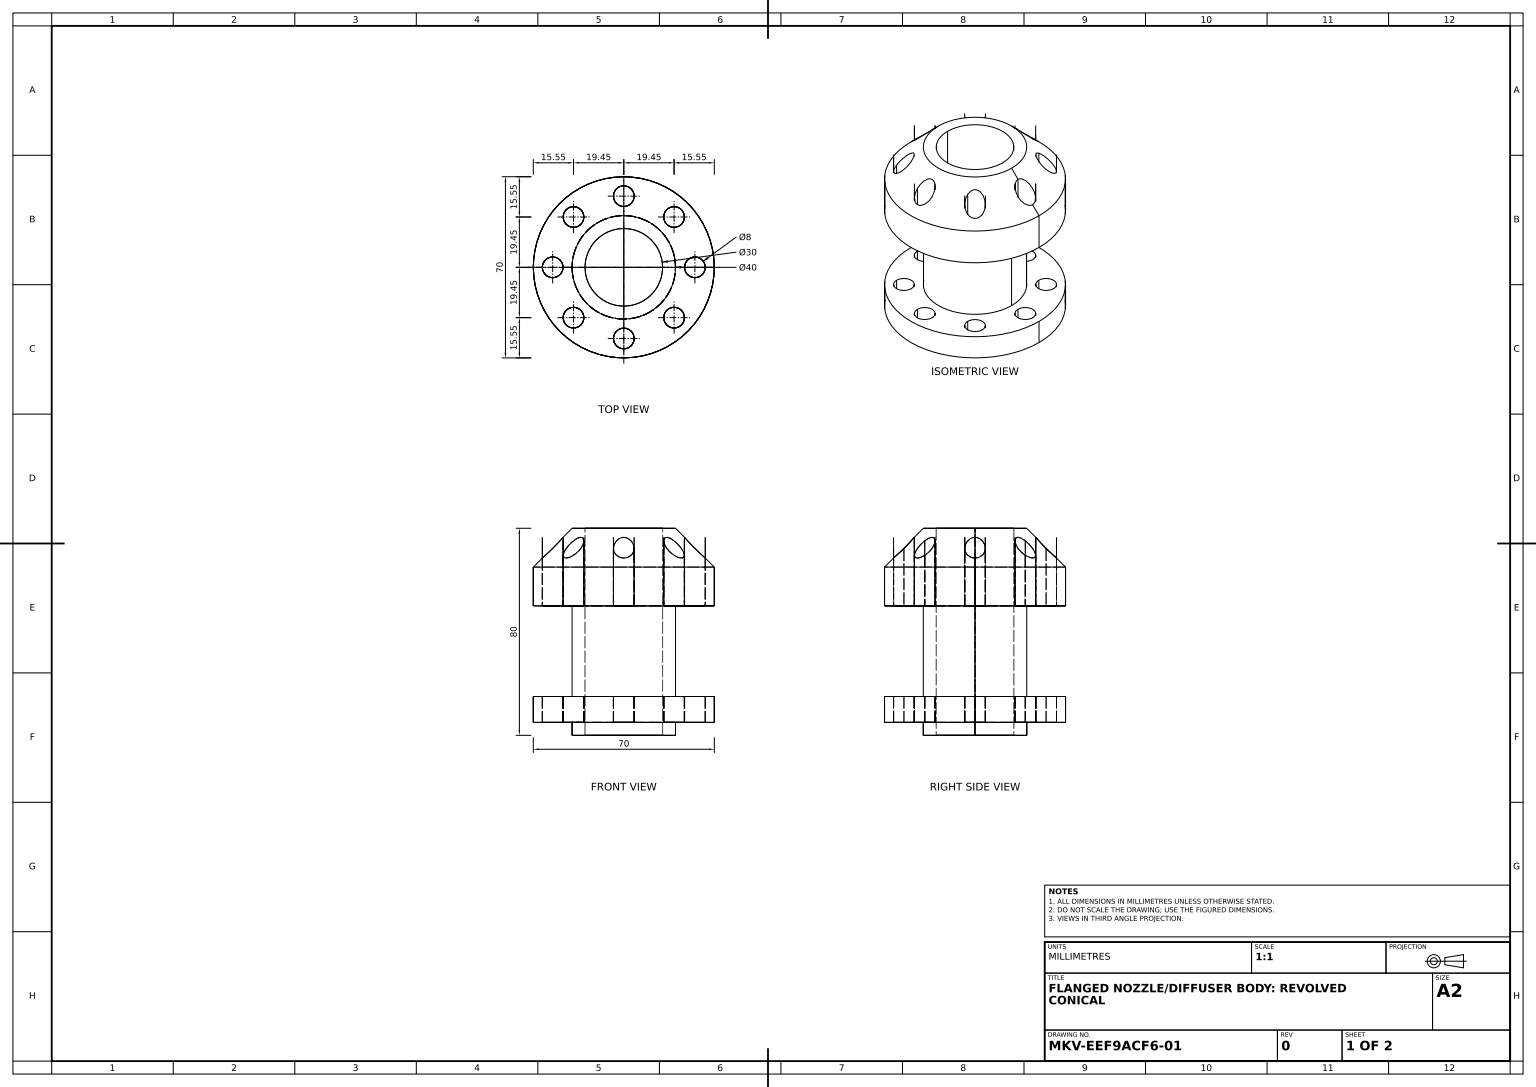
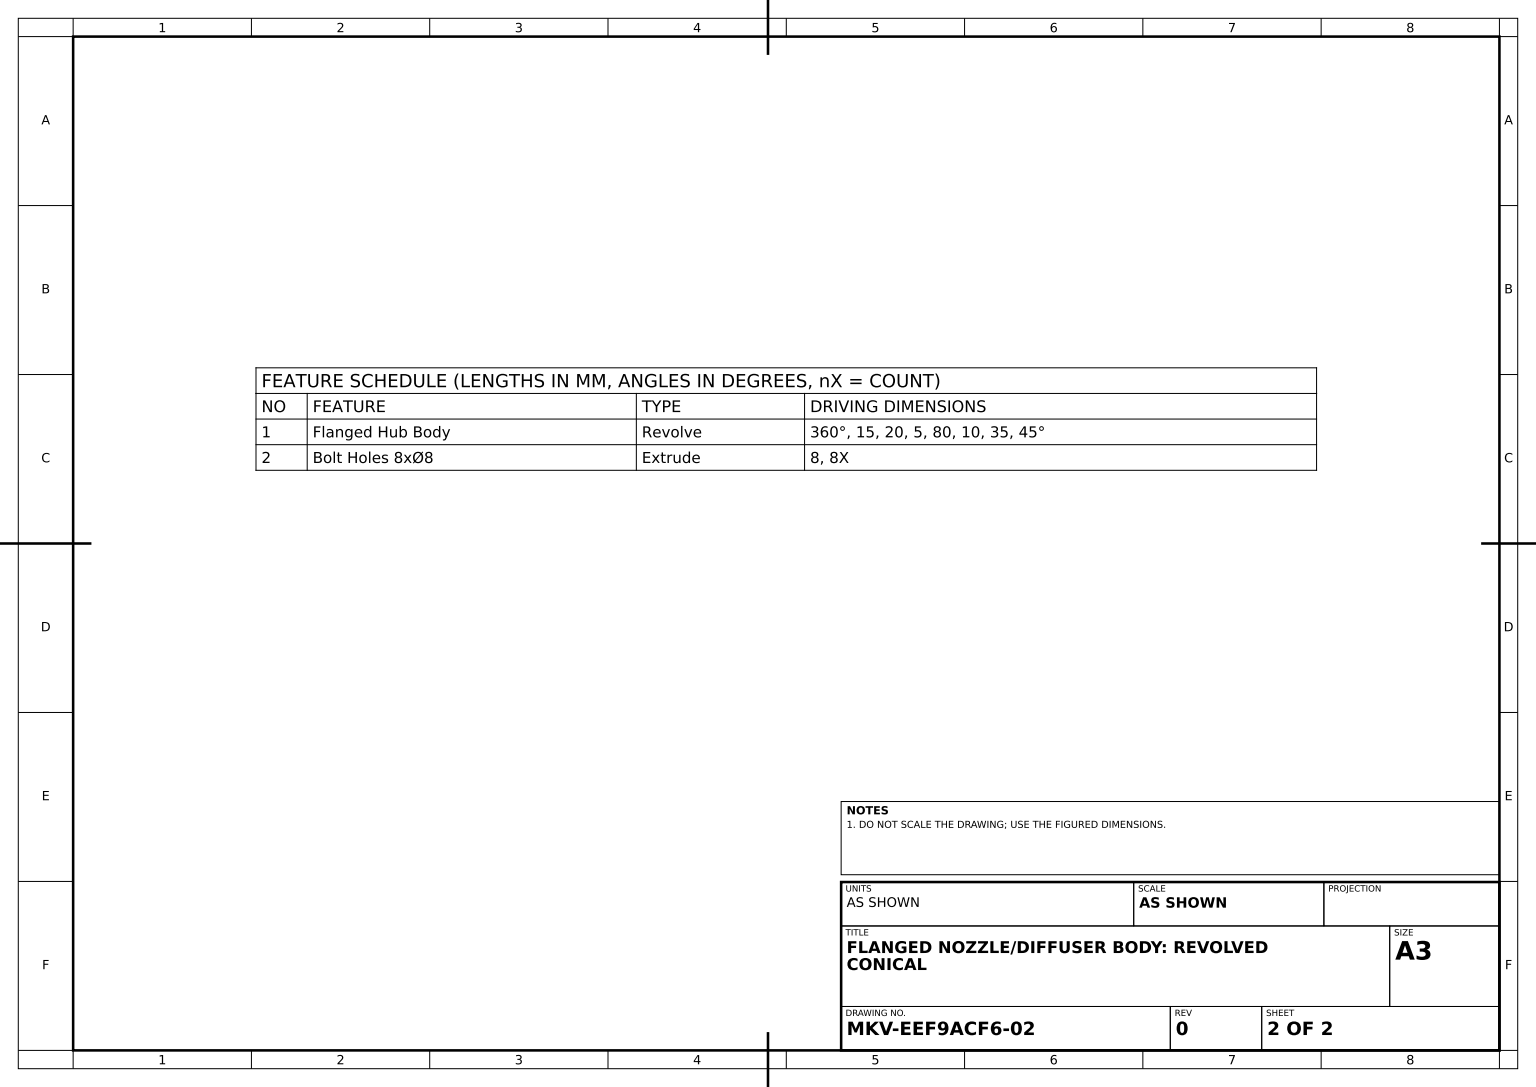
from build123d import *

# Parameters (mm, degrees)
BOLT_HOLES_8X_8_DEPTH      = 90.861003778
BOLT_HOLES_8X_8_DEPTH_BACK = 90.861003778
BOLT_HOLE_CIRCLE_SKETCH_R  = 4


with BuildPart() as part:
    # Hub Profile Sketch → Flanged Hub Body (revolve)
    with BuildSketch(Plane.XY):
        Polygon((-15, 40), (-15, -40), (-20, -40), (-20, -35), (-35, -35), (-35, -25), (-20, -25), (-20, 10), (-35, 10), (-35, 25), (-20, 40), align=None)
    revolve(axis=Axis((0, 43.460526316, 0), (0, -1, 0)))

    # Bolt Hole Circle Sketch → Bolt Holes 8xØ8 (cut, two sides: drawn at the far end of the back side and taken through both)
    with BuildSketch(Plane.XZ.offset(35).offset(-BOLT_HOLES_8X_8_DEPTH_BACK)):
        with Locations((27.5, 0)):
            Circle(BOLT_HOLE_CIRCLE_SKETCH_R)
        with Locations((19.445436483, -19.445436483)):
            Circle(BOLT_HOLE_CIRCLE_SKETCH_R)
        with Locations((0, -27.5)):
            Circle(BOLT_HOLE_CIRCLE_SKETCH_R)
        with Locations((-19.445436483, -19.445436483)):
            Circle(BOLT_HOLE_CIRCLE_SKETCH_R)
        with Locations((-27.5, 0)):
            Circle(BOLT_HOLE_CIRCLE_SKETCH_R)
        with Locations((-19.445436483, 19.445436483)):
            Circle(BOLT_HOLE_CIRCLE_SKETCH_R)
        with Locations((0, 27.5)):
            Circle(BOLT_HOLE_CIRCLE_SKETCH_R)
        with Locations((19.445436483, 19.445436483)):
            Circle(BOLT_HOLE_CIRCLE_SKETCH_R)
    extrude(amount=BOLT_HOLES_8X_8_DEPTH + BOLT_HOLES_8X_8_DEPTH_BACK, mode=Mode.SUBTRACT)


solid = part.part
